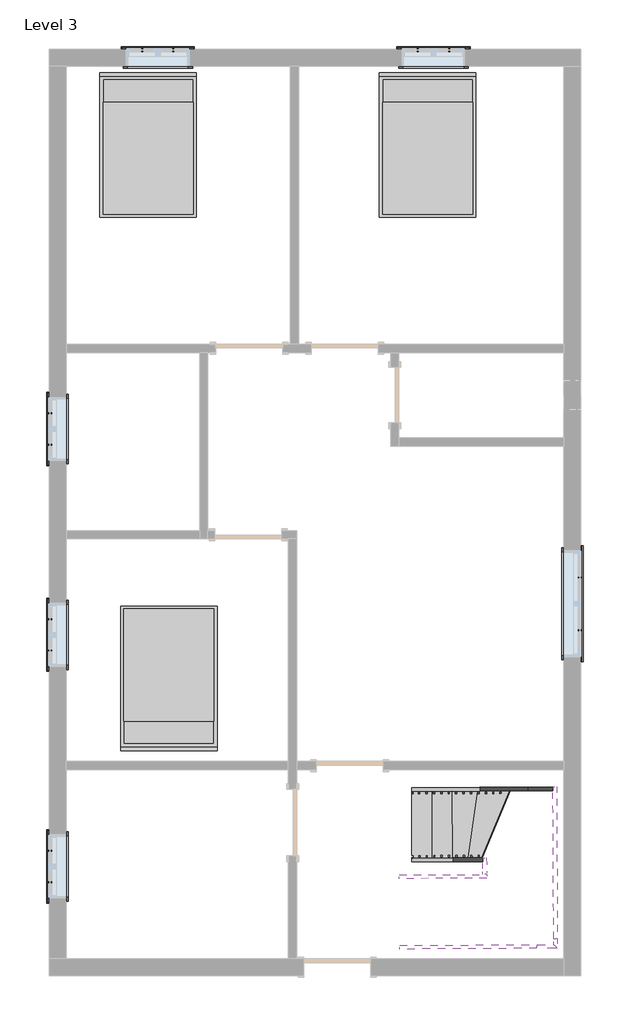
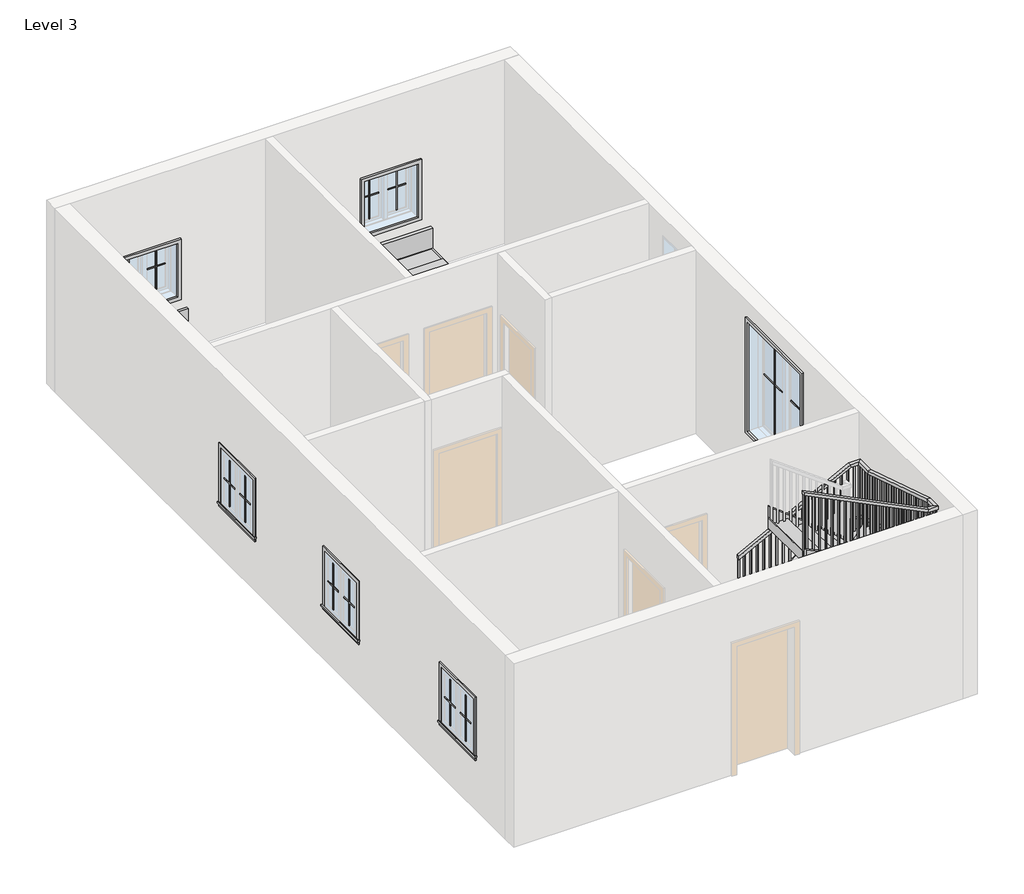
# One storey, part 2 of 2: 24 proxies, 9 members, 3 furniture elements, 1 railing, 1 stair flight.
"""IFC4 building model written with IfcOpenShell, lengths in millimetres."""

from ifc_helpers import new_model, si_unit, frame, origin, place, context, project, spatial, polyline, outline, extrude, faceted_brep, transform, mapped, element, save
from components import muntin_pattern_2x2_muntin_pattern_2x2_b3fe6957, muntin_pattern_2x2_muntin_pattern_2x2_3e0ecaf2, muntin_pattern_2x2_muntin_pattern_2x2_bff912c5, muntin_pattern_2x2_muntin_pattern_2x2_c2194282, trim_window_exterior_flat_with_sill_41619996, trim_window_exterior_flat_with_sill_e04b3088, trim_window_interior_flat_picture_frame_51c85655, trim_window_interior_flat_picture_frame_2a7685fe, bed_17739_bed_17739_15c61121, stair_flight_456e8720

model = new_model("IFC4")

# Units and contexts
model_context = context("Model", 3, world=origin())
ifc_project = project(units=[si_unit("LENGTHUNIT", "METRE", prefix="MILLI")], contexts=[model_context])

# Site, building, storey
site = spatial("IfcSite", under=ifc_project)
building = spatial("IfcBuilding", under=site)
storey = spatial("IfcBuildingStorey", under=building, Name="Level 3", Elevation=3200.4)

# Proxies
placement = place(None, origin())
muntin_pattern_2x2_muntin_pattern_2x2_shape = muntin_pattern_2x2_muntin_pattern_2x2_b3fe6957(model_context)
element("IfcBuildingElementProxy", 1, Name="Muntin Pattern_2x2 : Muntin Pattern_2x2", ObjectType="Muntin Pattern_2x2 : Muntin Pattern_2x2", at=placement, inside=storey, context=model_context, shape_type="MappedRepresentation", body=[
    mapped(muntin_pattern_2x2_muntin_pattern_2x2_shape, transform((-3622.2040084, 6872.3185985, 4184.65), x_axis=(1.0, 0.0, 0.0), y_axis=(0.0, 1.0, 0.0), z_axis=(0.0, 0.0, 1.0))),
])
element("IfcBuildingElementProxy", 2, Name="Muntin Pattern_2x2 : Muntin Pattern_2x2", ObjectType="Muntin Pattern_2x2 : Muntin Pattern_2x2", at=placement, inside=storey, context=model_context, shape_type="MappedRepresentation", body=[
    mapped(muntin_pattern_2x2_muntin_pattern_2x2_shape, transform((152.8709916, 6872.3185985, 4184.65), x_axis=(1.0, 0.0, 0.0), y_axis=(0.0, 1.0, 0.0), z_axis=(0.0, 0.0, 1.0))),
])
element("IfcBuildingElementProxy", 3, Name="Muntin Pattern_2x2 : Muntin Pattern_2x2", ObjectType="Muntin Pattern_2x2 : Muntin Pattern_2x2", at=placement, inside=storey, context=model_context, shape_type="MappedRepresentation", body=[
    mapped(muntin_pattern_2x2_muntin_pattern_2x2_shape, transform((-4884.2665084, 1466.8810985, 4184.65), x_axis=(0.0, 1.0, 0.0), y_axis=(-1.0, 0.0, 0.0), z_axis=(0.0, 0.0, 1.0))),
])
element("IfcBuildingElementProxy", 4, Name="Muntin Pattern_2x2 : Muntin Pattern_2x2", ObjectType="Muntin Pattern_2x2 : Muntin Pattern_2x2", at=placement, inside=storey, context=model_context, shape_type="MappedRepresentation", body=[
    mapped(muntin_pattern_2x2_muntin_pattern_2x2_shape, transform((-4884.2665084, -1352.5189015, 4184.65), x_axis=(0.0, 1.0, 0.0), y_axis=(-1.0, 0.0, 0.0), z_axis=(0.0, 0.0, 1.0))),
])
element("IfcBuildingElementProxy", 5, Name="Muntin Pattern_2x2 : Muntin Pattern_2x2", ObjectType="Muntin Pattern_2x2 : Muntin Pattern_2x2", at=placement, inside=storey, context=model_context, shape_type="MappedRepresentation", body=[
    mapped(muntin_pattern_2x2_muntin_pattern_2x2_shape, transform((-4884.2665084, -4524.3439015, 4184.65), x_axis=(0.0, 1.0, 0.0), y_axis=(-1.0, 0.0, 0.0), z_axis=(0.0, 0.0, 1.0))),
])
muntin_pattern_2x2_muntin_pattern_2x2_2_shape = muntin_pattern_2x2_muntin_pattern_2x2_3e0ecaf2(model_context)
element("IfcBuildingElementProxy", 6, Name="Muntin Pattern_2x2 : Muntin Pattern_2x2", ObjectType="Muntin Pattern_2x2 : Muntin Pattern_2x2", at=placement, inside=storey, context=model_context, shape_type="MappedRepresentation", body=[
    mapped(muntin_pattern_2x2_muntin_pattern_2x2_2_shape, transform((-3193.5790084, 6872.3185985, 4184.65), x_axis=(-1.0, 0.0, 0.0), y_axis=(0.0, -1.0, 0.0), z_axis=(0.0, 0.0, 1.0))),
])
element("IfcBuildingElementProxy", 7, Name="Muntin Pattern_2x2 : Muntin Pattern_2x2", ObjectType="Muntin Pattern_2x2 : Muntin Pattern_2x2", at=placement, inside=storey, context=model_context, shape_type="MappedRepresentation", body=[
    mapped(muntin_pattern_2x2_muntin_pattern_2x2_2_shape, transform((581.4959916, 6872.3185985, 4184.65), x_axis=(-1.0, 0.0, 0.0), y_axis=(0.0, -1.0, 0.0), z_axis=(0.0, 0.0, 1.0))),
])
element("IfcBuildingElementProxy", 8, Name="Muntin Pattern_2x2 : Muntin Pattern_2x2", ObjectType="Muntin Pattern_2x2 : Muntin Pattern_2x2", at=placement, inside=storey, context=model_context, shape_type="MappedRepresentation", body=[
    mapped(muntin_pattern_2x2_muntin_pattern_2x2_2_shape, transform((-4884.2665084, 1895.5060985, 4184.65), x_axis=(0.0, -1.0, 0.0), y_axis=(1.0, 0.0, 0.0), z_axis=(0.0, 0.0, 1.0))),
])
element("IfcBuildingElementProxy", 9, Name="Muntin Pattern_2x2 : Muntin Pattern_2x2", ObjectType="Muntin Pattern_2x2 : Muntin Pattern_2x2", at=placement, inside=storey, context=model_context, shape_type="MappedRepresentation", body=[
    mapped(muntin_pattern_2x2_muntin_pattern_2x2_2_shape, transform((-4884.2665084, -923.8939015, 4184.65), x_axis=(0.0, -1.0, 0.0), y_axis=(1.0, 0.0, 0.0), z_axis=(0.0, 0.0, 1.0))),
])
element("IfcBuildingElementProxy", 10, Name="Muntin Pattern_2x2 : Muntin Pattern_2x2", ObjectType="Muntin Pattern_2x2 : Muntin Pattern_2x2", at=placement, inside=storey, context=model_context, shape_type="MappedRepresentation", body=[
    mapped(muntin_pattern_2x2_muntin_pattern_2x2_2_shape, transform((-4884.2665084, -4095.7189015, 4184.65), x_axis=(0.0, -1.0, 0.0), y_axis=(1.0, 0.0, 0.0), z_axis=(0.0, 0.0, 1.0))),
])
muntin_pattern_2x2_muntin_pattern_2x2_3_shape = muntin_pattern_2x2_muntin_pattern_2x2_bff912c5(model_context)
element("IfcBuildingElementProxy", 11, Name="Muntin Pattern_2x2 : Muntin Pattern_2x2", ObjectType="Muntin Pattern_2x2 : Muntin Pattern_2x2", at=placement, inside=storey, context=model_context, shape_type="MappedRepresentation", body=[
    mapped(muntin_pattern_2x2_muntin_pattern_2x2_3_shape, transform((2373.7834916, -352.3939015, 4184.65), x_axis=(0.0, -1.0, 0.0), y_axis=(1.0, 0.0, 0.0), z_axis=(0.0, 0.0, 1.0))),
])
muntin_pattern_2x2_muntin_pattern_2x2_4_shape = muntin_pattern_2x2_muntin_pattern_2x2_c2194282(model_context)
element("IfcBuildingElementProxy", 12, Name="Muntin Pattern_2x2 : Muntin Pattern_2x2", ObjectType="Muntin Pattern_2x2 : Muntin Pattern_2x2", at=placement, inside=storey, context=model_context, shape_type="MappedRepresentation", body=[
    mapped(muntin_pattern_2x2_muntin_pattern_2x2_4_shape, transform((2373.7834916, -1073.1189015, 4184.65), x_axis=(0.0, 1.0, 0.0), y_axis=(-1.0, 0.0, 0.0), z_axis=(0.0, 0.0, 1.0))),
])
trim_window_exterior_flat_with_sill_shape = trim_window_exterior_flat_with_sill_41619996(model_context)
element("IfcBuildingElementProxy", 13, Name="Trim-Window-Exterior-Flat : with Sill", ObjectType="Trim-Window-Exterior-Flat : with Sill", at=placement, inside=storey, context=model_context, shape_type="MappedRepresentation", body=[
    mapped(trim_window_exterior_flat_with_sill_shape, transform((-3407.8915084, 6881.8435985, 5029.2), x_axis=(-1.0, 0.0, 0.0), y_axis=(0.0, 0.0, 1.0), z_axis=(0.0, 1.0, 0.0))),
])
element("IfcBuildingElementProxy", 14, Name="Trim-Window-Exterior-Flat : with Sill", ObjectType="Trim-Window-Exterior-Flat : with Sill", at=placement, inside=storey, context=model_context, shape_type="MappedRepresentation", body=[
    mapped(trim_window_exterior_flat_with_sill_shape, transform((367.1834916, 6881.8435985, 5029.2), x_axis=(-1.0, 0.0, 0.0), y_axis=(0.0, 0.0, 1.0), z_axis=(0.0, 1.0, 0.0))),
])
element("IfcBuildingElementProxy", 15, Name="Trim-Window-Exterior-Flat : with Sill", ObjectType="Trim-Window-Exterior-Flat : with Sill", at=placement, inside=storey, context=model_context, shape_type="MappedRepresentation", body=[
    mapped(trim_window_exterior_flat_with_sill_shape, transform((-4893.7915084, 1681.1935985, 5029.2), x_axis=(0.0, -1.0, 0.0), y_axis=(0.0, 0.0, 1.0), z_axis=(-1.0, 0.0, 0.0))),
])
element("IfcBuildingElementProxy", 16, Name="Trim-Window-Exterior-Flat : with Sill", ObjectType="Trim-Window-Exterior-Flat : with Sill", at=placement, inside=storey, context=model_context, shape_type="MappedRepresentation", body=[
    mapped(trim_window_exterior_flat_with_sill_shape, transform((-4893.7915084, -1138.2064015, 5029.2), x_axis=(0.0, -1.0, 0.0), y_axis=(0.0, 0.0, 1.0), z_axis=(-1.0, 0.0, 0.0))),
])
element("IfcBuildingElementProxy", 17, Name="Trim-Window-Exterior-Flat : with Sill", ObjectType="Trim-Window-Exterior-Flat : with Sill", at=placement, inside=storey, context=model_context, shape_type="MappedRepresentation", body=[
    mapped(trim_window_exterior_flat_with_sill_shape, transform((-4893.7915084, -4310.0314015, 5029.2), x_axis=(0.0, -1.0, 0.0), y_axis=(0.0, 0.0, 1.0), z_axis=(-1.0, 0.0, 0.0))),
])
trim_window_exterior_flat_with_sill_2_shape = trim_window_exterior_flat_with_sill_e04b3088(model_context)
element("IfcBuildingElementProxy", 18, Name="Trim-Window-Exterior-Flat : with Sill", ObjectType="Trim-Window-Exterior-Flat : with Sill", at=placement, inside=storey, context=model_context, shape_type="MappedRepresentation", body=[
    mapped(trim_window_exterior_flat_with_sill_2_shape, transform((2383.3084916, -712.7564015, 5943.6), x_axis=(0.0, 1.0, 0.0), y_axis=(0.0, 0.0, 1.0), z_axis=(1.0, 0.0, 0.0))),
])
trim_window_interior_flat_picture_frame_shape = trim_window_interior_flat_picture_frame_51c85655(model_context)
element("IfcBuildingElementProxy", 19, Name="Trim-Window-Interior-Flat : Picture Frame", ObjectType="Trim-Window-Interior-Flat : Picture Frame", at=placement, inside=storey, context=model_context, shape_type="MappedRepresentation", body=[
    mapped(trim_window_interior_flat_picture_frame_shape, transform((-3407.8915084, 6653.2435985, 5029.2), x_axis=(1.0, 0.0, 0.0), y_axis=(0.0, 0.0, 1.0), z_axis=(0.0, -1.0, 0.0))),
])
element("IfcBuildingElementProxy", 20, Name="Trim-Window-Interior-Flat : Picture Frame", ObjectType="Trim-Window-Interior-Flat : Picture Frame", at=placement, inside=storey, context=model_context, shape_type="MappedRepresentation", body=[
    mapped(trim_window_interior_flat_picture_frame_shape, transform((367.1834916, 6653.2435985, 5029.2), x_axis=(1.0, 0.0, 0.0), y_axis=(0.0, 0.0, 1.0), z_axis=(0.0, -1.0, 0.0))),
])
element("IfcBuildingElementProxy", 21, Name="Trim-Window-Interior-Flat : Picture Frame", ObjectType="Trim-Window-Interior-Flat : Picture Frame", at=placement, inside=storey, context=model_context, shape_type="MappedRepresentation", body=[
    mapped(trim_window_interior_flat_picture_frame_shape, transform((-4665.1915084, 1681.1935985, 5029.2), x_axis=(0.0, 1.0, 0.0), y_axis=(0.0, 0.0, 1.0), z_axis=(1.0, 0.0, 0.0))),
])
element("IfcBuildingElementProxy", 22, Name="Trim-Window-Interior-Flat : Picture Frame", ObjectType="Trim-Window-Interior-Flat : Picture Frame", at=placement, inside=storey, context=model_context, shape_type="MappedRepresentation", body=[
    mapped(trim_window_interior_flat_picture_frame_shape, transform((-4665.1915084, -1138.2064015, 5029.2), x_axis=(0.0, 1.0, 0.0), y_axis=(0.0, 0.0, 1.0), z_axis=(1.0, 0.0, 0.0))),
])
element("IfcBuildingElementProxy", 23, Name="Trim-Window-Interior-Flat : Picture Frame", ObjectType="Trim-Window-Interior-Flat : Picture Frame", at=placement, inside=storey, context=model_context, shape_type="MappedRepresentation", body=[
    mapped(trim_window_interior_flat_picture_frame_shape, transform((-4665.1915084, -4310.0314015, 5029.2), x_axis=(0.0, 1.0, 0.0), y_axis=(0.0, 0.0, 1.0), z_axis=(1.0, 0.0, 0.0))),
])
trim_window_interior_flat_picture_frame_2_shape = trim_window_interior_flat_picture_frame_2a7685fe(model_context)
element("IfcBuildingElementProxy", 24, Name="Trim-Window-Interior-Flat : Picture Frame", ObjectType="Trim-Window-Interior-Flat : Picture Frame", at=placement, inside=storey, context=model_context, shape_type="MappedRepresentation", body=[
    mapped(trim_window_interior_flat_picture_frame_2_shape, transform((2154.7084916, -712.7564015, 5943.6), x_axis=(0.0, -1.0, 0.0), y_axis=(0.0, 0.0, 1.0), z_axis=(-1.0, 0.0, 0.0))),
])

# Furniture
bed_17739_bed_17739_shape = bed_17739_bed_17739_15c61121(model_context)
element("IfcFurniture", 25, ObjectType="Bed_17739 : Bed_17739", at=placement, inside=storey, context=model_context, shape_type="MappedRepresentation", body=[
    mapped(bed_17739_bed_17739_shape, transform((-3541.2415084, 5548.3435985, 3200.4), x_axis=(1.0, 0.0, 0.0), y_axis=(0.0, 1.0, 0.0), z_axis=(0.0, 0.0, 1.0))),
])
element("IfcFurniture", 26, ObjectType="Bed_17739 : Bed_17739", at=placement, inside=storey, context=model_context, shape_type="MappedRepresentation", body=[
    mapped(bed_17739_bed_17739_shape, transform((287.8084916, 5548.3435985, 3200.4), x_axis=(1.0, 0.0, 0.0), y_axis=(0.0, 1.0, 0.0), z_axis=(0.0, 0.0, 1.0))),
])
element("IfcFurniture", 27, ObjectType="Bed_17739 : Bed_17739", at=placement, inside=storey, context=model_context, shape_type="MappedRepresentation", body=[
    mapped(bed_17739_bed_17739_shape, transform((-3255.4915084, -1709.7064015, 3200.4), x_axis=(-1.0, 0.0, 0.0), y_axis=(0.0, -1.0, 0.0), z_axis=(0.0, 0.0, 1.0))),
])

# Members
element("IfcMember", 28, ObjectType="Stringer - 2\" Width", at=placement, inside=storey, context=model_context, shape_type="SweptSolid", body=[
    extrude(outline(polyline([(149.3129896, -304.8), (0.0, 0.0), (1768.8429208, 0.0), (1918.1559104, -304.8000001), (149.3129896, -304.8)])), frame((68.8012135, -3282.7418259, 3603.7997735), z_axis=(-0.00516207396967135, 0.9999866764074069, 0.0), x_axis=(0.8980237466183223, 0.004635726771100007, 0.4399225619889199)), (0.0, 0.0, 1.0), 50.8),
])
element("IfcMember", 29, ObjectType="Stringer - 2\" Width", at=placement, inside=storey, context=model_context, shape_type="SweptSolid", body=[
    extrude(outline(polyline([(1657.2641604, -3274.5419534), (1657.0019271, -3223.7426303), (2003.5241973, -3221.9538329), (2003.7864306, -3272.753156), (1657.2641604, -3274.5419534)])), frame((0.0, 0.0, 4381.953683), z_axis=(0.0, 0.0, 1.0), x_axis=(1.0, 0.0, 0.0)), (0.0, 0.0, 1.0), 339.4074379),
])
element("IfcMember", 30, ObjectType="Stringer - 2\" Width", at=placement, inside=storey, context=model_context, shape_type="SweptSolid", body=[
    extrude(outline(polyline([(47.2049979, -324.2228076), (-38.2916769, -48.0839082), (117.0107078, 0.0), (2125.7436964, 0.0), (2226.1278582, -324.2228076), (47.2049979, -324.2228076)])), frame((2003.7864306, -3272.753156, 4381.953683), z_axis=(0.9999866764074068, 0.005162073969671772, 0.0), x_axis=(0.0049311297532716285, -0.9552486233011704, 0.295762999106675)), (0.0, 0.0, 1.0), 50.8),
])
element("IfcMember", 31, ObjectType="Stringer - 2\" Width", at=placement, inside=storey, context=model_context, shape_type="SweptSolid", body=[
    extrude(outline(polyline([(2014.2687486, -5303.3668955), (2065.0680718, -5303.1046621), (2065.7306715, -5431.462157), (2014.669115, -5380.9250672), (2014.2687486, -5303.3668955)])), frame((0.0, 0.0, 5020.6291102), z_axis=(0.0, 0.0, 1.0), x_axis=(1.0, 0.0, 0.0)), (0.0, 0.0, 1.0), 319.0749838),
])
element("IfcMember", 32, ObjectType="Stringer - 2\" Width", at=placement, inside=storey, context=model_context, shape_type="SweptSolid", body=[
    extrude(outline(polyline([(2014.669115, -5380.9250672), (2065.7306715, -5431.462157), (1782.4368375, -5432.9245602), (1782.1746041, -5382.1252371), (2014.669115, -5380.9250672)])), frame((0.0, 0.0, 5020.6291102), z_axis=(0.0, 0.0, 1.0), x_axis=(1.0, 0.0, 0.0)), (0.0, 0.0, 1.0), 319.0749838),
])
element("IfcMember", 33, ObjectType="Stringer - 2\" Width", at=placement, inside=storey, context=model_context, shape_type="SweptSolid", body=[
    extrude(outline(polyline([(286.8047106, -304.8), (0.0, 0.0), (1331.6484515, 0.0), (1618.4531621, -304.8), (286.8047106, -304.8)])), frame((73.7836473, -4247.928966, 3446.9616111), z_axis=(-0.005162073969671482, 0.9999866764074068, 0.0), x_axis=(0.7282688430294204, 0.0037594277266083504, 0.6852812261953175)), (0.0, 0.0, 1.0), 50.8),
])
element("IfcMember", 34, ObjectType="Stringer - 2\" Width", at=placement, inside=storey, context=model_context, shape_type="SweptSolid", body=[
    extrude(outline(polyline([(660.780085, -304.8), (110.7389009, -51.080863), (134.3011229, 0.0), (545.7678218, 0.0), (1125.9670058, -267.6302075), (1108.8215849, -304.8), (660.780085, -304.8)])), frame((1043.319491, -4192.1234067, 4285.3637993), z_axis=(0.9999866764074068, 0.005162073969671282, 0.0), x_axis=(0.002162183372020065, -0.4188538515087163, 0.90805108669027)), (0.0, 0.0, 1.0), 50.8),
])
element("IfcMember", 35, ObjectType="Stringer - 2\" Width", at=placement, inside=storey, context=model_context, shape_type="SweptSolid", body=[
    extrude(outline(polyline([(-239.6623642, -304.8), (0.0, 0.0), (1521.9461582, 0.0), (1282.2837939, -304.8), (-239.6623642, -304.8)])), frame((1095.5610976, -4471.2574507, 5419.8987993), z_axis=(-0.005162073969672184, 0.9999866764074068, 0.0), x_axis=(-0.7860864868637559, -0.0040578906574323574, 0.6181032023000775)), (0.0, 0.0, 1.0), 50.8),
])
element("IfcMember", 36, ObjectType="Stringer - 2\" Width", at=placement, inside=storey, context=model_context, shape_type="SweptSolid", body=[
    extrude(outline(polyline([(-137.2719745, -288.0368905), (0.0, 0.0), (2080.7002403, 0.0), (1943.4282658, -288.0368905), (-137.2719745, -288.0368905)])), frame((1782.4368375, -5432.9245602, 5339.704094), z_axis=(-0.005162073969672376, 0.9999866764074068, 0.0), x_axis=(-0.9027127399072911, -0.004659932023802854, 0.43021854242071556)), (0.0, 0.0, 1.0), 50.8),
])

# Railing
element("IfcRailing", 37, ObjectType="Handrail - Rectangular", at=placement, inside=storey, context=model_context, shape_type="SolidModel", body=[
    faceted_brep([(68.8012135, -3282.7418259, 4792.1333333), (68.8012135, -3282.7418259, 4735.0032367), (69.0634468, -3333.5411491, 4735.0032367), (69.0634468, -3333.5411491, 4792.1333333), (1818.9474855, -3273.707321, 5692.6523232), (1831.2499413, -3273.643814, 5641.8523232), (1831.5121746, -3324.4431372, 5641.8523232), (1819.2097188, -3324.5066442, 5692.6523232), (2003.7864306, -3272.753156, 5692.6523232), (2003.7864306, -3272.753156, 5641.8523232), (1953.2493408, -3323.8147125, 5641.8523232), (1953.2493408, -3323.8147125, 5692.6523232), (2005.285328, -3563.1165554, 5692.6523232), (2005.3249947, -3570.8007251, 5641.8523232), (1954.5256716, -3571.0629585, 5641.8523232), (1954.4860048, -3563.3787887, 5692.6523232), (2013.5123671, -5156.842168, 6186.0998462), (2013.5520339, -5164.5263378, 6135.2998462), (1962.7527107, -5164.7885712, 6135.2998462), (1962.7130439, -5157.1044014, 6186.0998462), (2014.669115, -5380.9250672, 6186.0998462), (2014.669115, -5380.9250672, 6135.2998462), (1963.6075585, -5330.3879774, 6135.2998462), (1963.6075585, -5330.3879774, 6186.0998462), (1865.7077622, -5381.694027, 6186.0998462), (1853.7618085, -5381.7556937, 6135.2998462), (1853.4995752, -5330.9563705, 6135.2998462), (1865.4455288, -5330.8947038, 6186.0998462), (-96.1000106, -5391.8211588, 7162.8), (-96.362244, -5341.0218356, 7162.8), (-96.362244, -5341.0218356, 7106.0526208), (-96.1000106, -5391.8211588, 7106.0526208)], [[[0, 1, 2, 3]], [[1, 0, 4, 5]], [[2, 1, 5, 6]], [[3, 2, 6, 7]], [[0, 3, 7, 4]], [[5, 4, 8, 9]], [[6, 5, 9, 10]], [[7, 6, 10, 11]], [[4, 7, 11, 8]], [[9, 8, 12, 13]], [[10, 9, 13, 14]], [[11, 10, 14, 15]], [[8, 11, 15, 12]], [[13, 12, 16, 17]], [[14, 13, 17, 18]], [[15, 14, 18, 19]], [[12, 15, 19, 16]], [[17, 16, 20, 21]], [[18, 17, 21, 22]], [[19, 18, 22, 23]], [[16, 19, 23, 20]], [[21, 20, 24, 25]], [[22, 21, 25, 26]], [[23, 22, 26, 27]], [[20, 23, 27, 24]], [[28, 29, 30, 31]], [[25, 24, 28, 31]], [[26, 25, 31, 30]], [[27, 26, 30, 29]], [[24, 27, 29, 28]]]),
    extrude(outline(polyline([(223.8579732, 19.05), (1229.0021026, 19.05), (1229.0021026, 0.0), (233.3420268, 0.0), (223.8579732, 19.05)])), frame((-33.2605479, -5375.621561, 7308.0687693), z_axis=(-0.005162073969671937, 0.9999866764074068, 0.0), x_axis=(0.0, 0.0, -1.0)), (0.0, 0.0, 1.0), 19.05),
    extrude(outline(polyline([(223.8579732, 19.0499999), (1178.4204835, 19.0499999), (1178.4204835, 0.0), (233.3420268, 0.0), (223.8579732, 19.0499999)])), frame((68.3380984, -5375.0970942, 7257.4871502), z_axis=(-0.005162073969671937, 0.9999866764074068, 0.0), x_axis=(0.0, 0.0, -1.0)), (0.0, 0.0, 1.0), 19.05),
    extrude(outline(polyline([(223.8579732, 19.05), (1127.8388644, 19.05), (1127.8388644, 0.0), (233.3420268, 0.0), (223.8579732, 19.05)])), frame((169.9367448, -5374.5726275, 7206.9055311), z_axis=(-0.005162073969671937, 0.9999866764074068, 0.0), x_axis=(0.0, 0.0, -1.0)), (0.0, 0.0, 1.0), 19.05),
    extrude(outline(polyline([(223.8579732, 19.05), (1246.5905787, 19.05), (1246.5905787, 0.0), (233.3420268, 0.0), (223.8579732, 19.05)])), frame((271.5353911, -5374.0481608, 7156.323912), z_axis=(-0.005162073969671937, 0.9999866764074068, 0.0), x_axis=(0.0, 0.0, -1.0)), (0.0, 0.0, 1.0), 19.05),
    extrude(outline(polyline([(223.8579732, 19.05), (1196.0089596, 19.05), (1196.0089596, 0.0), (233.3420267, 0.0), (223.8579732, 19.05)])), frame((373.1340374, -5373.5236941, 7105.7422929), z_axis=(-0.005162073969671937, 0.9999866764074068, 0.0), x_axis=(0.0, 0.0, -1.0)), (0.0, 0.0, 1.0), 19.05),
    extrude(outline(polyline([(223.8579732, 19.05), (1314.7606738, 19.05), (1314.7606738, 0.0), (233.3420267, 0.0), (223.8579732, 19.05)])), frame((474.7326837, -5372.9992274, 7055.1606738), z_axis=(-0.005162073969671937, 0.9999866764074068, 0.0), x_axis=(0.0, 0.0, -1.0)), (0.0, 0.0, 1.0), 19.05),
    extrude(outline(polyline([(223.8579733, 19.05), (1264.1790548, 19.05), (1264.1790548, 0.0), (233.3420268, 0.0), (223.8579733, 19.05)])), frame((576.3313301, -5372.4747607, 7004.5790548), z_axis=(-0.005162073969671937, 0.9999866764074068, 0.0), x_axis=(0.0, 0.0, -1.0)), (0.0, 0.0, 1.0), 19.05),
    extrude(outline(polyline([(223.8579732, 19.05), (1213.5974357, 19.05), (1213.5974357, 0.0), (233.3420268, 0.0), (223.8579732, 19.05)])), frame((677.9299764, -5371.950294, 6953.9974357), z_axis=(-0.005162073969671937, 0.9999866764074068, 0.0), x_axis=(0.0, 0.0, -1.0)), (0.0, 0.0, 1.0), 19.05),
    extrude(outline(polyline([(223.8579732, 19.05), (1163.0158166, 19.05), (1163.0158166, 0.0), (233.3420268, 0.0), (223.8579732, 19.05)])), frame((779.5286227, -5371.4258272, 6903.4158166), z_axis=(-0.005162073969671937, 0.9999866764074068, 0.0), x_axis=(0.0, 0.0, -1.0)), (0.0, 0.0, 1.0), 19.05),
    extrude(outline(polyline([(223.8579732, 19.05), (1281.7675308, 19.05), (1281.7675308, 0.0), (233.3420268, 0.0), (223.8579732, 19.05)])), frame((881.127269, -5370.9013605, 6852.8341975), z_axis=(-0.005162073969671937, 0.9999866764074068, 0.0), x_axis=(0.0, 0.0, -1.0)), (0.0, 0.0, 1.0), 19.05),
    extrude(outline(polyline([(223.8579732, 19.0499999), (1231.1859117, 19.0499999), (1231.1859117, 0.0), (233.3420268, 0.0), (223.8579732, 19.0499999)])), frame((982.7259153, -5370.3768938, 6802.2525784), z_axis=(-0.005162073969671937, 0.9999866764074068, 0.0), x_axis=(0.0, 0.0, -1.0)), (0.0, 0.0, 1.0), 19.05),
    extrude(outline(polyline([(223.8579732, 19.05), (1180.6042926, 19.05), (1180.6042926, 0.0), (233.3420268, 0.0), (223.8579732, 19.05)])), frame((1084.3245617, -5369.8524271, 6751.6709593), z_axis=(-0.005162073969671937, 0.9999866764074068, 0.0), x_axis=(0.0, 0.0, -1.0)), (0.0, 0.0, 1.0), 19.05),
    extrude(outline(polyline([(223.8579732, 19.05), (1299.3560069, 19.05), (1299.3560069, 0.0), (233.3420268, 0.0), (223.8579732, 19.05)])), frame((1185.923208, -5369.3279604, 6701.0893402), z_axis=(-0.005162073969671937, 0.9999866764074068, 0.0), x_axis=(0.0, 0.0, -1.0)), (0.0, 0.0, 1.0), 19.05),
    extrude(outline(polyline([(223.8579732, 19.05), (1248.7743878, 19.05), (1248.7743878, 0.0), (233.3420268, 0.0), (223.8579732, 19.05)])), frame((1287.5218543, -5368.8034937, 6650.5077211), z_axis=(-0.005162073969671937, 0.9999866764074068, 0.0), x_axis=(0.0, 0.0, -1.0)), (0.0, 0.0, 1.0), 19.05),
    extrude(outline(polyline([(223.8579732, 19.0499999), (1198.1927687, 19.0499999), (1198.1927687, 0.0), (233.3420268, 0.0), (223.8579732, 19.0499999)])), frame((1389.1205006, -5368.2790269, 6599.926102), z_axis=(-0.005162073969671937, 0.9999866764074068, 0.0), x_axis=(0.0, 0.0, -1.0)), (0.0, 0.0, 1.0), 19.05),
    extrude(outline(polyline([(223.8579732, 19.05), (1147.6111496, 19.05), (1147.6111496, 0.0), (233.3420268, 0.0), (223.8579732, 19.05)])), frame((1490.719147, -5367.7545602, 6549.3444829), z_axis=(-0.005162073969671937, 0.9999866764074068, 0.0), x_axis=(0.0, 0.0, -1.0)), (0.0, 0.0, 1.0), 19.05),
    extrude(outline(polyline([(223.8579732, 19.05), (1097.0295305, 19.05), (1097.0295305, 0.0), (233.3420267, 0.0), (223.8579732, 19.05)])), frame((1592.3177933, -5367.2300935, 6498.7628638), z_axis=(-0.005162073969671937, 0.9999866764074068, 0.0), x_axis=(0.0, 0.0, -1.0)), (0.0, 0.0, 1.0), 19.05),
    extrude(outline(polyline([(223.8579733, 19.05), (1215.7812448, 19.05), (1215.7812448, 0.0), (233.3420268, 0.0), (223.8579733, 19.05)])), frame((1693.9164396, -5366.7056268, 6448.1812448), z_axis=(-0.005162073969671937, 0.9999866764074068, 0.0), x_axis=(0.0, 0.0, -1.0)), (0.0, 0.0, 1.0), 19.05),
    extrude(outline(polyline([(223.8579733, 19.05), (1165.1996257, 19.05), (1165.1996257, 0.0), (233.3420268, 0.0), (223.8579733, 19.05)])), frame((1795.5150859, -5366.1811601, 6397.5996257), z_axis=(-0.005162073969671937, 0.9999866764074068, 0.0), x_axis=(0.0, 0.0, -1.0)), (0.0, 0.0, 1.0), 19.05),
    extrude(outline(polyline([(1897.1137323, -5365.6566934), (1878.0639861, -5365.7550309), (1877.9656486, -5346.7052847), (1897.0153947, -5346.6069472), (1897.1137323, -5365.6566934)])), frame((0.0, 0.0, 5232.4), z_axis=(0.0, 0.0, 1.0), x_axis=(1.0, 0.0, 0.0)), (0.0, 0.0, 1.0), 902.8998462),
    extrude(outline(polyline([(1998.4829244, -5320.6828189), (1998.5812619, -5339.7325651), (1979.5315157, -5339.8309026), (1979.4331782, -5320.7811564), (1998.4829244, -5320.6828189)])), frame((0.0, 0.0, 5232.4), z_axis=(0.0, 0.0, 1.0), x_axis=(1.0, 0.0, 0.0)), (0.0, 0.0, 1.0), 902.8998462),
    extrude(outline(polyline([(1997.9584577, -5219.0841726), (1998.0567952, -5238.1339187), (1979.007049, -5238.2322563), (1978.9087115, -5219.1825101), (1997.9584577, -5219.0841726)])), frame((0.0, 0.0, 5232.4), z_axis=(0.0, 0.0, 1.0), x_axis=(1.0, 0.0, 0.0)), (0.0, 0.0, 1.0), 902.8998462),
    extrude(outline(polyline([(231.5490805, 19.05), (1119.8588311, 19.05), (1119.8588311, 0.0), (225.6509196, 0.0), (231.5490805, 19.05)])), frame((1978.4825823, -5136.6336099, 6352.2588311), z_axis=(0.9999866764074068, 0.005162073969671697, 0.0), x_axis=(0.0, 0.0, -1.0)), (0.0, 0.0, 1.0), 19.05),
    extrude(outline(polyline([(231.5490804, 19.05), (1088.401973, 19.05), (1088.401973, 0.0), (225.6509195, 0.0), (231.5490804, 19.05)])), frame((1977.9581156, -5035.0349636, 6320.801973), z_axis=(0.9999866764074068, 0.005162073969671697, 0.0), x_axis=(0.0, 0.0, -1.0)), (0.0, 0.0, 1.0), 19.05),
    extrude(outline(polyline([(231.5490805, 19.05), (1226.2784483, 19.05), (1226.2784483, 0.0), (225.6509196, 0.0), (231.5490805, 19.05)])), frame((1977.4336488, -4933.4363173, 6289.345115), z_axis=(0.9999866764074068, 0.005162073969671697, 0.0), x_axis=(0.0, 0.0, -1.0)), (0.0, 0.0, 1.0), 19.05),
    extrude(outline(polyline([(231.5490804, 19.05), (1194.8215902, 19.05), (1194.8215902, 0.0), (225.6509195, 0.0), (231.5490804, 19.05)])), frame((1976.9091821, -4831.837671, 6257.8882569), z_axis=(0.9999866764074068, 0.005162073969671697, 0.0), x_axis=(0.0, 0.0, -1.0)), (0.0, 0.0, 1.0), 19.05),
    extrude(outline(polyline([(231.5490805, 19.0499999), (1163.3647322, 19.0499999), (1163.3647322, 0.0), (225.6509196, 0.0), (231.5490805, 19.0499999)])), frame((1976.3847154, -4730.2390246, 6226.4313989), z_axis=(0.9999866764074068, 0.005162073969671697, 0.0), x_axis=(0.0, 0.0, -1.0)), (0.0, 0.0, 1.0), 19.05),
    extrude(outline(polyline([(231.5490804, 19.05), (1131.9078741, 19.05), (1131.9078741, 0.0), (225.6509195, 0.0), (231.5490804, 19.05)])), frame((1975.8602487, -4628.6403783, 6194.9745408), z_axis=(0.9999866764074068, 0.005162073969671697, 0.0), x_axis=(0.0, 0.0, -1.0)), (0.0, 0.0, 1.0), 19.05),
    extrude(outline(polyline([(231.5490805, 19.05), (1100.4510161, 19.05), (1100.4510161, 0.0), (225.6509196, 0.0), (231.5490805, 19.05)])), frame((1975.335782, -4527.041732, 6163.5176828), z_axis=(0.9999866764074068, 0.005162073969671697, 0.0), x_axis=(0.0, 0.0, -1.0)), (0.0, 0.0, 1.0), 19.05),
    extrude(outline(polyline([(231.5490804, 19.05), (1238.3274914, 19.05), (1238.3274914, 0.0), (225.6509195, 0.0), (231.5490804, 19.05)])), frame((1974.8113153, -4425.4430857, 6132.0608247), z_axis=(0.9999866764074068, 0.005162073969671697, 0.0), x_axis=(0.0, 0.0, -1.0)), (0.0, 0.0, 1.0), 19.05),
    extrude(outline(polyline([(231.5490805, 19.05), (1206.8706334, 19.05), (1206.8706334, 0.0), (225.6509196, 0.0), (231.5490805, 19.05)])), frame((1974.2868486, -4323.8444394, 6100.6039667), z_axis=(0.9999866764074068, 0.005162073969671697, 0.0), x_axis=(0.0, 0.0, -1.0)), (0.0, 0.0, 1.0), 19.05),
    extrude(outline(polyline([(231.5490804, 19.05), (1175.4137753, 19.05), (1175.4137753, 0.0), (225.6509195, 0.0), (231.5490804, 19.05)])), frame((1973.7623818, -4222.245793, 6069.1471086), z_axis=(0.9999866764074068, 0.005162073969671697, 0.0), x_axis=(0.0, 0.0, -1.0)), (0.0, 0.0, 1.0), 19.05),
    extrude(outline(polyline([(231.5490804, 19.05), (1143.9569173, 19.05), (1143.9569173, 0.0), (225.6509196, 0.0), (231.5490804, 19.05)])), frame((1973.2379151, -4120.6471467, 6037.6902506), z_axis=(0.9999866764074068, 0.005162073969671697, 0.0), x_axis=(0.0, 0.0, -1.0)), (0.0, 0.0, 1.0), 19.05),
    extrude(outline(polyline([(231.5490805, 19.05), (1281.8333926, 19.05), (1281.8333926, 0.0), (225.6509196, 0.0), (231.5490805, 19.05)])), frame((1972.7134484, -4019.0485004, 6006.2333926), z_axis=(0.9999866764074068, 0.005162073969671697, 0.0), x_axis=(0.0, 0.0, -1.0)), (0.0, 0.0, 1.0), 19.05),
    extrude(outline(polyline([(231.5490804, 19.05), (1250.3765345, 19.05), (1250.3765345, 0.0), (225.6509196, 0.0), (231.5490804, 19.05)])), frame((1972.1889817, -3917.4498541, 5974.7765345), z_axis=(0.9999866764074068, 0.005162073969671697, 0.0), x_axis=(0.0, 0.0, -1.0)), (0.0, 0.0, 1.0), 19.05),
    extrude(outline(polyline([(231.5490805, 19.0499999), (1218.9196765, 19.0499999), (1218.9196765, 0.0), (225.6509196, 0.0), (231.5490805, 19.0499999)])), frame((1971.664515, -3815.8512077, 5943.3196765), z_axis=(0.9999866764074068, 0.005162073969671697, 0.0), x_axis=(0.0, 0.0, -1.0)), (0.0, 0.0, 1.0), 19.05),
    extrude(outline(polyline([(231.5490804, 19.05), (1187.4628184, 19.05), (1187.4628184, 0.0), (225.6509195, 0.0), (231.5490804, 19.05)])), frame((1971.1400483, -3714.2525614, 5911.8628184), z_axis=(0.9999866764074068, 0.005162073969671697, 0.0), x_axis=(0.0, 0.0, -1.0)), (0.0, 0.0, 1.0), 19.05),
    extrude(outline(polyline([(231.5490805, 19.05), (1156.0059604, 19.05), (1156.0059604, 0.0), (225.6509196, 0.0), (231.5490805, 19.05)])), frame((1970.6155816, -3612.6539151, 5880.4059604), z_axis=(0.9999866764074068, 0.005162073969671697, 0.0), x_axis=(0.0, 0.0, -1.0)), (0.0, 0.0, 1.0), 19.05),
    extrude(outline(polyline([(1989.0425235, -3491.9071851), (1989.140861, -3510.9569313), (1970.0911148, -3511.0552688), (1969.9927773, -3492.0055226), (1989.0425235, -3491.9071851)])), frame((0.0, 0.0, 4724.4), z_axis=(0.0, 0.0, 1.0), x_axis=(1.0, 0.0, 0.0)), (0.0, 0.0, 1.0), 917.4523232),
    extrude(outline(polyline([(1988.5180568, -3390.3085387), (1988.6163943, -3409.3582849), (1969.5666481, -3409.4566224), (1969.4683106, -3390.4068763), (1988.5180568, -3390.3085387)])), frame((0.0, 0.0, 4555.0666667), z_axis=(0.0, 0.0, 1.0), x_axis=(1.0, 0.0, 0.0)), (0.0, 0.0, 1.0), 1086.7856565),
    extrude(outline(polyline([(1888.1339221, -3289.2253823), (1907.1836683, -3289.1270448), (1907.2820058, -3308.176791), (1888.2322596, -3308.2751285), (1888.1339221, -3289.2253823)])), frame((0.0, 0.0, 4555.0666667), z_axis=(0.0, 0.0, 1.0), x_axis=(1.0, 0.0, 0.0)), (0.0, 0.0, 1.0), 1086.7856565),
    extrude(outline(polyline([(233.5009213, 19.05), (1297.2369609, 19.05), (1297.2369609, 0.0), (223.6990787, 0.0), (233.5009213, 19.05)])), frame((1805.6833595, -3308.7012577, 5852.3036276), z_axis=(-0.005162073969671542, 0.9999866764074069, 0.0), x_axis=(0.0, 0.0, -1.0)), (0.0, 0.0, 1.0), 19.05),
    extrude(outline(polyline([(233.5009213, 19.05), (1244.9604673, 19.05), (1244.9604673, 0.0), (223.6990787, 0.0), (233.5009213, 19.05)])), frame((1704.0847132, -3309.2257244, 5800.027134), z_axis=(-0.005162073969671542, 0.9999866764074069, 0.0), x_axis=(0.0, 0.0, -1.0)), (0.0, 0.0, 1.0), 19.05),
    extrude(outline(polyline([(233.5009212, 19.05), (1192.6839737, 19.05), (1192.6839737, 0.0), (223.6990787, 0.0), (233.5009212, 19.05)])), frame((1602.4860668, -3309.7501911, 5747.7506404), z_axis=(-0.005162073969671542, 0.9999866764074069, 0.0), x_axis=(0.0, 0.0, -1.0)), (0.0, 0.0, 1.0), 19.05),
    extrude(outline(polyline([(233.5009212, 19.05), (1140.4074801, 19.05), (1140.4074801, 0.0), (223.6990787, 0.0), (233.5009212, 19.05)])), frame((1500.8874205, -3310.2746578, 5695.4741468), z_axis=(-0.005162073969671542, 0.9999866764074069, 0.0), x_axis=(0.0, 0.0, -1.0)), (0.0, 0.0, 1.0), 19.05),
    extrude(outline(polyline([(233.5009213, 19.05), (1088.1309866, 19.05), (1088.1309866, 0.0), (223.6990788, 0.0), (233.5009213, 19.05)])), frame((1399.2887742, -3310.7991245, 5643.1976533), z_axis=(-0.005162073969671542, 0.9999866764074069, 0.0), x_axis=(0.0, 0.0, -1.0)), (0.0, 0.0, 1.0), 19.05),
    extrude(outline(polyline([(233.5009213, 19.05), (1205.1878264, 19.05), (1205.1878264, 0.0), (223.6990788, 0.0), (233.5009213, 19.05)])), frame((1297.6901279, -3311.3235913, 5590.9211597), z_axis=(-0.005162073969671542, 0.9999866764074069, 0.0), x_axis=(0.0, 0.0, -1.0)), (0.0, 0.0, 1.0), 19.05),
    extrude(outline(polyline([(233.5009213, 19.0499999), (1152.9113328, 19.0499999), (1152.9113328, 0.0), (223.6990787, 0.0), (233.5009213, 19.0499999)])), frame((1196.0914815, -3311.848058, 5538.6446661), z_axis=(-0.005162073969671542, 0.9999866764074069, 0.0), x_axis=(0.0, 0.0, -1.0)), (0.0, 0.0, 1.0), 19.05),
    extrude(outline(polyline([(233.5009213, 19.05), (1100.6348392, 19.05), (1100.6348392, 0.0), (223.6990787, 0.0), (233.5009213, 19.05)])), frame((1094.4928352, -3312.3725247, 5486.3681725), z_axis=(-0.005162073969671542, 0.9999866764074069, 0.0), x_axis=(0.0, 0.0, -1.0)), (0.0, 0.0, 1.0), 19.05),
    extrude(outline(polyline([(233.5009213, 19.05), (1048.3583456, 19.05), (1048.3583456, 0.0), (223.6990787, 0.0), (233.5009213, 19.05)])), frame((992.8941889, -3312.8969914, 5434.0916789), z_axis=(-0.005162073969671542, 0.9999866764074069, 0.0), x_axis=(0.0, 0.0, -1.0)), (0.0, 0.0, 1.0), 19.05),
    extrude(outline(polyline([(233.5009212, 19.05), (1165.4151853, 19.05), (1165.4151853, 0.0), (223.6990787, 0.0), (233.5009212, 19.05)])), frame((891.2955426, -3313.4214581, 5381.8151853), z_axis=(-0.005162073969671542, 0.9999866764074069, 0.0), x_axis=(0.0, 0.0, -1.0)), (0.0, 0.0, 1.0), 19.05),
    extrude(outline(polyline([(233.5009213, 19.0499999), (1113.1386918, 19.0499999), (1113.1386918, 0.0), (223.6990788, 0.0), (233.5009213, 19.0499999)])), frame((789.6968962, -3313.9459248, 5329.5386918), z_axis=(-0.005162073969671542, 0.9999866764074069, 0.0), x_axis=(0.0, 0.0, -1.0)), (0.0, 0.0, 1.0), 19.05),
    extrude(outline(polyline([(233.5009213, 19.05), (1060.8621982, 19.05), (1060.8621982, 0.0), (223.6990788, 0.0), (233.5009213, 19.05)])), frame((688.0982499, -3314.4703915, 5277.2621982), z_axis=(-0.005162073969671542, 0.9999866764074069, 0.0), x_axis=(0.0, 0.0, -1.0)), (0.0, 0.0, 1.0), 19.05),
    extrude(outline(polyline([(233.5009213, 19.05), (1177.9190379, 19.05), (1177.9190379, 0.0), (223.6990787, 0.0), (233.5009213, 19.05)])), frame((586.4996036, -3314.9948583, 5224.9857046), z_axis=(-0.005162073969671542, 0.9999866764074069, 0.0), x_axis=(0.0, 0.0, -1.0)), (0.0, 0.0, 1.0), 19.05),
    extrude(outline(polyline([(233.5009213, 19.05), (1125.6425443, 19.05), (1125.6425443, 0.0), (223.6990787, 0.0), (233.5009213, 19.05)])), frame((484.9009573, -3315.519325, 5172.709211), z_axis=(-0.005162073969671542, 0.9999866764074069, 0.0), x_axis=(0.0, 0.0, -1.0)), (0.0, 0.0, 1.0), 19.05),
    extrude(outline(polyline([(233.5009213, 19.05), (1073.3660507, 19.05), (1073.3660507, 0.0), (223.6990787, 0.0), (233.5009213, 19.05)])), frame((383.302311, -3316.0437917, 5120.4327174), z_axis=(-0.005162073969671542, 0.9999866764074069, 0.0), x_axis=(0.0, 0.0, -1.0)), (0.0, 0.0, 1.0), 19.05),
    extrude(outline(polyline([(233.5009212, 19.05), (1190.4228905, 19.05), (1190.4228905, 0.0), (223.6990787, 0.0), (233.5009212, 19.05)])), frame((281.7036646, -3316.5682584, 5068.1562238), z_axis=(-0.005162073969671542, 0.9999866764074069, 0.0), x_axis=(0.0, 0.0, -1.0)), (0.0, 0.0, 1.0), 19.05),
    extrude(outline(polyline([(233.5009212, 19.05), (1138.1463969, 19.05), (1138.1463969, 0.0), (223.6990787, 0.0), (233.5009212, 19.05)])), frame((180.1050183, -3317.0927251, 5015.8797302), z_axis=(-0.005162073969671542, 0.9999866764074069, 0.0), x_axis=(0.0, 0.0, -1.0)), (0.0, 0.0, 1.0), 19.05),
    extrude(outline(polyline([(1998.6140411, -5346.0824805), (1998.7123786, -5365.1322267), (1979.6626324, -5365.2305642), (1979.5642949, -5346.180818), (1998.6140411, -5346.0824805)])), frame((0.0, 0.0, 5232.4), z_axis=(0.0, 0.0, 1.0), x_axis=(1.0, 0.0, 0.0)), (0.0, 0.0, 1.0), 902.8998462),
    extrude(outline(polyline([(1968.9438439, -3288.8082299), (1987.9935901, -3288.7098924), (1988.0919276, -3307.7596386), (1969.0421814, -3307.8579761), (1968.9438439, -3288.8082299)])), frame((0.0, 0.0, 4555.0666667), z_axis=(0.0, 0.0, 1.0), x_axis=(1.0, 0.0, 0.0)), (0.0, 0.0, 1.0), 1086.7856565),
    extrude(outline(polyline([(223.8579732, 19.05), (1250.8439273, 19.05), (1250.8439273, 0.0), (233.3420268, 0.0), (223.8579732, 19.05)])), frame((-77.1322124, -5375.8480328, 7329.910594), z_axis=(-0.005162073969671937, 0.9999866764074068, 0.0), x_axis=(0.0, 0.0, -1.0)), (0.0, 0.0, 1.0), 19.05),
    extrude(outline(polyline([(233.5009212, 19.05), (1090.7708246, 19.05), (1090.7708246, 0.0), (223.6990787, 0.0), (233.5009212, 19.05)])), frame((88.0312451, -3317.5680231, 4968.5041579), z_axis=(-0.005162073969671542, 0.9999866764074069, 0.0), x_axis=(0.0, 0.0, -1.0)), (0.0, 0.0, 1.0), 19.05),
])

# Stair flight
stair_flight_shape = stair_flight_456e8720(model_context)
element("IfcStairFlight", 38, ObjectType="2\" Tread 1\" Nosing 1/4\" Riser", at=placement, inside=storey, context=model_context, shape_type="MappedRepresentation", body=[
    mapped(stair_flight_shape, transform((0.0, 0.0, 0.0), x_axis=(1.0, 0.0, 0.0), y_axis=(0.0, 1.0, 0.0), z_axis=(0.0, 0.0, 1.0))),
])

save(model, "model.ifc")

# Revit data of these elements
# Type "Muntin Pattern_2x2 : Muntin Pattern_2x2"
#   Width [instance default] = 4' - 0"
#   Thickness = 0' - 0 1/2"
#   Height [instance default] = 4' - 0"
#   Distance = 0' - 0 3/4"
#   Interior Material [instance default] = none
#   Exterior Material [instance default] = none
#   Default Elevation = 0
# Type "Trim-Window-Exterior-Flat : with Sill"
#   Trim Width = 0' - 2 1/4"
#   Trim Thickness_Picture Frame = 0' - 1 1/4"
#   Trim Thickness_with Sill = 0' - 0 3/4"
#   Sill Thickness = 0' - 1 1/4"
#   Opening Width [instance default] = 2' - 0"
#   Opening Height [instance default] = 3' - 0"
#   Default Elevation = 4' - 0"
#   Sill = yes
#   Picture Frame = no
#   Trim Material [instance default] = none
# Type "Trim-Window-Interior-Flat : Picture Frame"
#   Trim Thickness_Picture Frame = 0' - 1 1/4"
#   Trim Width = 0' - 2 1/4"
#   Trim Thickness_with Sill = 0' - 0 3/4"
#   Sill Thickness = 0' - 1 1/4"
#   Opening Width [instance default] = 2' - 0"
#   Opening Height [instance default] = 3' - 0"
#   Default Elevation = 4' - 0"
#   Sill = no
#   Picture Frame = yes
#   Trim Material [instance default] = none
# Type "Bed_17739 : Bed_17739"
#   Default Elevation = 0
# Type "Handrail - Rectangular"
#   Assembly Code = "C2010400"
#   built-in parameter 1008612 = 0.0416667 (stored number, unit not read)
#   built-in parameter 1008611 = 0.0416667 (stored number, unit not read)
#   built-in parameter 1008609 = 0.333333 (stored number, unit not read)
#   built-in parameter 1008604 = 0.166667 (stored number, unit not read)
#   built-in parameter 1008603 = 0.166667 (stored number, unit not read)
#   Railing Height = 3' - 0"
#   built-in parameter 1008630 = 2
#   built-in parameter 1008610 = 2
#   built-in parameter 1008618 = Baluster - Square : 3/4"
# Elements 1, 2, 3, 4, 5, 6, 7, 8, 9, 10 (IfcBuildingElementProxy, "Muntin Pattern_2x2 : Muntin Pattern_2x2")
#   Width = 0' - 11 5/8"
#   Height = 2' - 6 1/2"
#   Interior Material = Wood - Stained
#   Exterior Material = Clad - White
#   Phase Created = New Construction
#   Materials on its faces: "Clad - White", "Wood - Stained"
# Elements 11, 12 (IfcBuildingElementProxy, "Muntin Pattern_2x2 : Muntin Pattern_2x2")
#   Width = 1' - 11 1/8"
#   Height = 5' - 6 1/2"
#   Interior Material = Wood - Stained
#   Exterior Material = Clad - White
#   Phase Created = New Construction
#   Materials on its faces: "Clad - White", "Wood - Stained"
# Elements 13, 14, 15, 16, 17 (IfcBuildingElementProxy, "Trim-Window-Exterior-Flat : with Sill")
#   Opening Width = 2' - 10"
#   Opening Height = 3' - 0"
#   Trim Material = Clad - White
#   Phase Created = New Construction
#   Materials on its faces: "Clad - White"
# Element 18 (IfcBuildingElementProxy, "Trim-Window-Exterior-Flat : with Sill")
#   Opening Width = 4' - 9"
#   Opening Height = 6' - 0"
#   Trim Material = Clad - White
#   Phase Created = New Construction
#   Materials on its faces: "Clad - White"
# Elements 19, 20, 21, 22, 23 (IfcBuildingElementProxy, "Trim-Window-Interior-Flat : Picture Frame")
#   Opening Width = 2' - 10"
#   Opening Height = 3' - 0"
#   Trim Material = Wood - Stained
#   Phase Created = New Construction
#   Materials on its faces: "Wood - Stained"
# Element 24 (IfcBuildingElementProxy, "Trim-Window-Interior-Flat : Picture Frame")
#   Opening Width = 4' - 9"
#   Opening Height = 6' - 0"
#   Trim Material = Wood - Stained
#   Phase Created = New Construction
#   Materials on its faces: "Wood - Stained"
# Elements 25, 26, 27 (IfcFurniture, "Bed_17739 : Bed_17739")
#   Phase Created = New Construction
#   Materials on its faces: "legs", "sheets", "bed frame", "Blanket"
# Elements 28, 29, 30, 31, 32, 33, 34, 35, 36 (IfcMember, "Stringer - 2\" Width")
#   Phase Created = New Construction
# Element 37 (IfcRailing, "Handrail - Rectangular")
#   Phase Created = New Construction
# Element 38 (IfcStairFlight, "2\" Tread 1\" Nosing 1/4\" Riser")
#   Phase Created = New Construction
# Materials
#   "Clad - White": class "Wood", colour RGB 242 242 238, transparency 0, Cost = 0
#   "Wood - Stained": class "Wood", colour RGB 224 178 126, transparency 0, Cost = 0
#   "legs": colour RGB 90 73 37, transparency 0, Cost = 0
#   "sheets": colour RGB 200 195 176, transparency 0, Cost = 0
#   "bed frame": colour RGB 90 73 37, transparency 0, Cost = 0
#   "Blanket": class "System", colour RGB 59 0 1, transparency 0, Cost = 0
